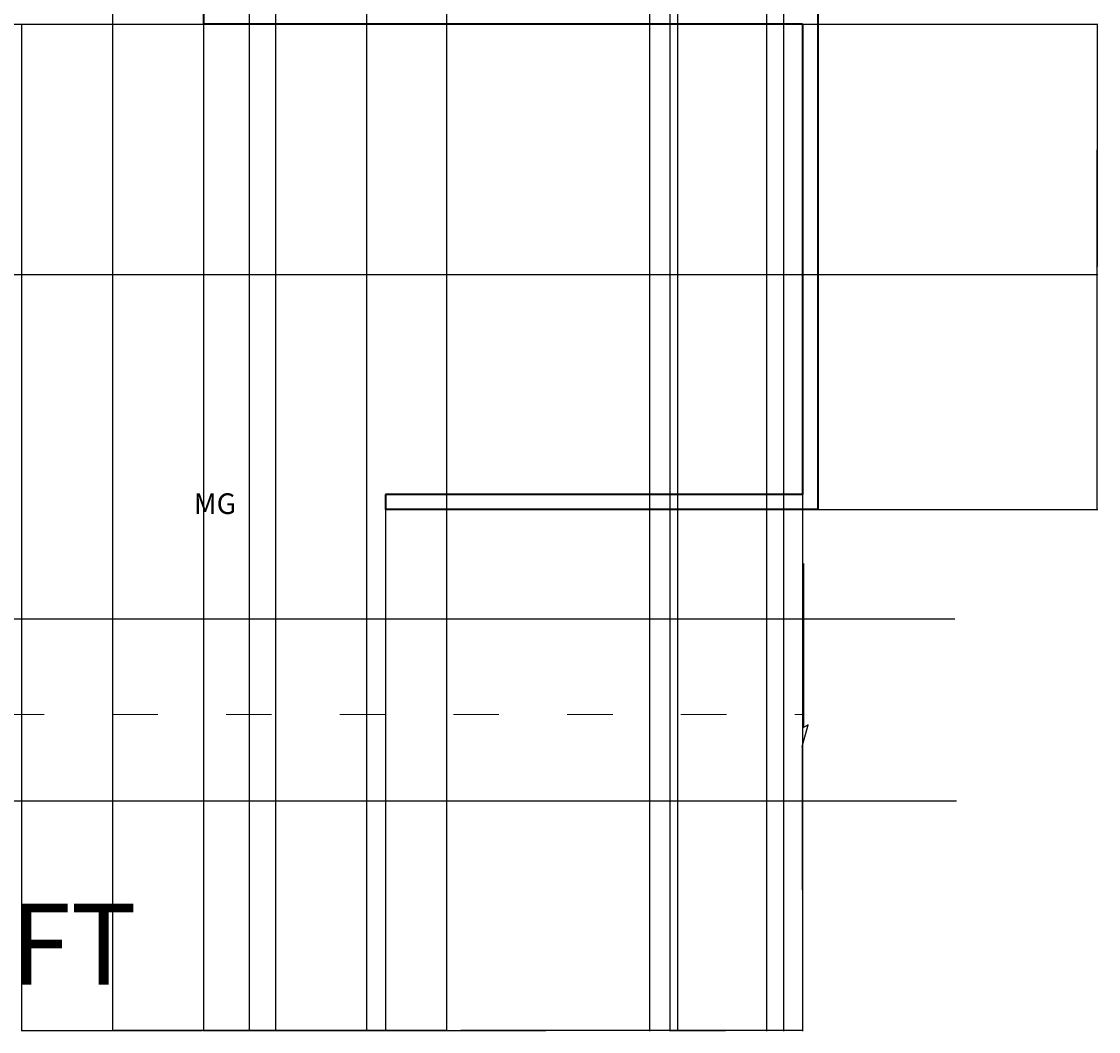
# Model space of a CAD drawing. Units: inches. Extents: x 320 to 1055, y -655 to 96.
# Tile 2 of 4: x 771 to 1055, y -655 to -389. Entities that reach past the tile are written whole.
import ezdxf

# ---------------------------------------------------------------- set-up
doc = ezdxf.new("R2010")
doc.units = ezdxf.units.IN
doc.header["$MEASUREMENT"] = 0
doc.linetypes.add('ACAD_ISO03W100', pattern=[30, 12, -18])
for name, color, linetype, lineweight in [('A-ANNO-DIMS', 2, 'Continuous', 18), ('A-ANNO-IDEN', 1, 'Continuous', 18), ('A-ANNO-TEXT', 8, 'Continuous', 18), ('C-ROAD', 1, 'Continuous', 25), ('C-ROAD-CNTR', 1, 'ACAD_ISO03W100', 18), ('wall', 1, 'Continuous', 35)]:
    doc.layers.add(name, color=color, linetype=linetype, lineweight=lineweight)
doc.styles.get("Standard").update_dxf_attribs({"font": 'arial.ttf'})
doc.dimstyles.get("Standard").update_dxf_attribs({"dimtxt": 0.18, "dimasz": 0.18, "dimexe": 0.18, "dimexo": 0.0625, "dimgap": 0.09, "dimtad": 0, "dimtih": 1, "dimtoh": 1, "dimdec": 1, "dimzin": 0, "dimdsep": 46, "dimlunit": 4, "dimtxsty": 'Standard', "dimcen": 0.09, "dimadec": 0, "dimazin": 0, "dimtfac": 1, "dimtdec": 1, "dimtofl": 0, "dimtmove": 0, "dimatfit": 3, "dimfxl": 1, "dimtolj": 1, "dimtzin": 0, "dimarcsym": 0})

# ---------------------------------------------------------------- blocks, each defined once
blk = doc.blocks.new('*D17')
at = {"layer": 'A-ANNO-DIMS', "color": 0, "lineweight": -2, "transparency": 16777216}
for p, q in [((770.86, -517.8), (770.86, -655.29)), ((866.86, -517.8), (866.86, -655.29)), ((771.04, -655.11), (818.53, -655.11)), ((866.68, -655.11), (819.19, -655.11))]:
    blk.add_line(p, q, dxfattribs=at)
at = {"layer": 'A-ANNO-DIMS', "color": 0, "transparency": 16777216}
for points in [[(771.04, -655.08), (771.04, -655.14), (770.86, -655.11)], [(866.68, -655.08), (866.68, -655.14), (866.86, -655.11)]]:
    blk.add_solid(points, dxfattribs=at)
at = {"layer": 'Defpoints', "color": 0, "transparency": 16777216}
for p in [(770.86, -517.74), (866.86, -517.74), (866.86, -655.11)]:
    blk.add_point(p, dxfattribs=at)
at = {"layer": 'A-ANNO-DIMS', "color": 0, "transparency": 16777216, "insert": (818.86, -655.11), "char_height": 0.18, "attachment_point": 5}
blk.add_mtext('\\A1;8\'-0"', dxfattribs=at)
blk = doc.blocks.new('*D18')
at = {"layer": 'A-ANNO-DIMS', "color": 0, "lineweight": -2, "transparency": 16777216}
for p, q in [((818.86, -389.8), (818.86, -655.29)), ((976.86, -389.8), (976.86, -655.29)), ((819.04, -655.11), (897.47, -655.11)), ((976.68, -655.11), (898.25, -655.11))]:
    blk.add_line(p, q, dxfattribs=at)
at = {"layer": 'A-ANNO-DIMS', "color": 0, "transparency": 16777216}
for points in [[(819.04, -655.08), (819.04, -655.14), (818.86, -655.11)], [(976.68, -655.08), (976.68, -655.14), (976.86, -655.11)]]:
    blk.add_solid(points, dxfattribs=at)
at = {"layer": 'Defpoints', "color": 0, "transparency": 16777216}
for p in [(818.86, -389.74), (976.86, -389.74), (976.86, -655.11)]:
    blk.add_point(p, dxfattribs=at)
at = {"layer": 'A-ANNO-DIMS', "color": 0, "transparency": 16777216, "insert": (897.86, -655.11), "char_height": 0.18, "attachment_point": 5}
blk.add_mtext('\\A1;13\'-2"', dxfattribs=at)
blk = doc.blocks.new('*D19')
at = {"layer": 'A-ANNO-DIMS', "color": 0, "lineweight": -2, "transparency": 16777216}
for p, q in [((976.92, -389.74), (1054.75, -389.74)), ((1054.57, -389.92), (1054.57, -453.55)), ((1054.57, -517.56), (1054.57, -453.92)), ((980.92, -517.74), (1054.75, -517.74))]:
    blk.add_line(p, q, dxfattribs=at)
at = {"layer": 'A-ANNO-DIMS', "color": 0, "transparency": 16777216}
for points in [[(1054.54, -389.92), (1054.6, -389.92), (1054.57, -389.74)], [(1054.54, -517.56), (1054.6, -517.56), (1054.57, -517.74)]]:
    blk.add_solid(points, dxfattribs=at)
at = {"layer": 'Defpoints', "color": 0, "transparency": 16777216}
for p in [(976.86, -389.74), (980.86, -517.74), (1054.57, -517.74)]:
    blk.add_point(p, dxfattribs=at)
at = {"layer": 'A-ANNO-DIMS', "color": 0, "transparency": 16777216, "insert": (1054.57, -453.74), "char_height": 0.18, "attachment_point": 5}
blk.add_mtext('\\A1;10\'-8"', dxfattribs=at)
blk = doc.blocks.new('*D20')
at = {"layer": 'A-ANNO-DIMS', "color": 0, "lineweight": -2, "transparency": 16777216}
for p, q in [((770.86, -389.8), (770.86, -655.29)), ((818.86, -389.8), (818.86, -655.29)), ((771.04, -655.11), (794.53, -655.11)), ((818.68, -655.11), (795.19, -655.11))]:
    blk.add_line(p, q, dxfattribs=at)
at = {"layer": 'A-ANNO-DIMS', "color": 0, "transparency": 16777216}
for points in [[(771.04, -655.08), (771.04, -655.14), (770.86, -655.11)], [(818.68, -655.08), (818.68, -655.14), (818.86, -655.11)]]:
    blk.add_solid(points, dxfattribs=at)
at = {"layer": 'Defpoints', "color": 0, "transparency": 16777216}
for p in [(770.86, -389.74), (818.86, -389.74), (818.86, -655.11)]:
    blk.add_point(p, dxfattribs=at)
at = {"layer": 'A-ANNO-DIMS', "color": 0, "transparency": 16777216, "insert": (794.86, -655.11), "char_height": 0.18, "attachment_point": 5}
blk.add_mtext('\\A1;4\'-0"', dxfattribs=at)
blk = doc.blocks.new('*D23')
at = {"layer": 'A-ANNO-DIMS', "color": 0, "lineweight": -2, "transparency": 16777216}
for p, q in [((794.86, -80.8), (794.86, -655.29)), ((818.86, -80.8), (818.86, -655.29)), ((795.04, -655.11), (806.53, -655.11)), ((818.68, -655.11), (807.19, -655.11))]:
    blk.add_line(p, q, dxfattribs=at)
at = {"layer": 'A-ANNO-DIMS', "color": 0, "transparency": 16777216}
for points in [[(795.04, -655.08), (795.04, -655.14), (794.86, -655.11)], [(818.68, -655.08), (818.68, -655.14), (818.86, -655.11)]]:
    blk.add_solid(points, dxfattribs=at)
at = {"layer": 'Defpoints', "color": 0, "transparency": 16777216}
for p in [(794.86, -80.74), (818.86, -80.74), (818.86, -655.11)]:
    blk.add_point(p, dxfattribs=at)
at = {"layer": 'A-ANNO-DIMS', "color": 0, "transparency": 16777216, "insert": (806.86, -655.11), "char_height": 0.18, "attachment_point": 5}
blk.add_mtext('\\A1;2\'-0"', dxfattribs=at)
blk = doc.blocks.new('*D25')
at = {"layer": 'A-ANNO-DIMS', "color": 0, "lineweight": -2, "transparency": 16777216}
for p, q in [((941.86, -380.8), (941.86, -655.29)), ((971.86, -380.8), (971.86, -655.29)), ((942.04, -655.11), (956.53, -655.11)), ((971.68, -655.11), (957.19, -655.11))]:
    blk.add_line(p, q, dxfattribs=at)
at = {"layer": 'A-ANNO-DIMS', "color": 0, "transparency": 16777216}
for points in [[(942.04, -655.08), (942.04, -655.14), (941.86, -655.11)], [(971.68, -655.08), (971.68, -655.14), (971.86, -655.11)]]:
    blk.add_solid(points, dxfattribs=at)
at = {"layer": 'Defpoints', "color": 0, "transparency": 16777216}
for p in [(941.86, -380.74), (971.86, -380.74), (941.86, -655.11)]:
    blk.add_point(p, dxfattribs=at)
at = {"layer": 'A-ANNO-DIMS', "color": 0, "transparency": 16777216, "insert": (956.86, -655.11), "char_height": 0.18, "attachment_point": 5}
blk.add_mtext('\\A1;2\'-6"', dxfattribs=at)
blk = doc.blocks.new('*D28')
at = {"layer": 'A-ANNO-DIMS', "color": 0, "lineweight": -2, "transparency": 16777216}
for p, q in [((943.86, -363.86), (943.86, -655.29)), ((967.33, -363.86), (967.33, -655.29)), ((944.04, -655.11), (955, -655.11)), ((967.15, -655.11), (956.2, -655.11))]:
    blk.add_line(p, q, dxfattribs=at)
at = {"layer": 'A-ANNO-DIMS', "color": 0, "transparency": 16777216}
for points in [[(944.04, -655.08), (944.04, -655.14), (943.86, -655.11)], [(967.15, -655.08), (967.15, -655.14), (967.33, -655.11)]]:
    blk.add_solid(points, dxfattribs=at)
at = {"layer": 'Defpoints', "color": 0, "transparency": 16777216}
for p in [(943.86, -363.79), (967.33, -363.79), (967.33, -655.11)]:
    blk.add_point(p, dxfattribs=at)
at = {"layer": 'A-ANNO-DIMS', "color": 0, "transparency": 16777216, "insert": (955.6, -655.11), "char_height": 0.18, "attachment_point": 5}
blk.add_mtext('\\A1;1\'-11 1/2"', dxfattribs=at)
blk = doc.blocks.new('*D30')
at = {"layer": 'A-ANNO-DIMS', "color": 0, "lineweight": -2, "transparency": 16777216}
for p, q in [((837.86, -248.8), (837.86, -655.29)), ((861.86, -248.8), (861.86, -655.29)), ((838.04, -655.11), (849.53, -655.11)), ((861.68, -655.11), (850.19, -655.11))]:
    blk.add_line(p, q, dxfattribs=at)
at = {"layer": 'A-ANNO-DIMS', "color": 0, "transparency": 16777216}
for points in [[(838.04, -655.08), (838.04, -655.14), (837.86, -655.11)], [(861.68, -655.08), (861.68, -655.14), (861.86, -655.11)]]:
    blk.add_solid(points, dxfattribs=at)
at = {"layer": 'Defpoints', "color": 0, "transparency": 16777216}
for p in [(837.86, -248.74), (861.86, -248.74), (861.86, -655.11)]:
    blk.add_point(p, dxfattribs=at)
at = {"layer": 'A-ANNO-DIMS', "color": 0, "transparency": 16777216, "insert": (849.86, -655.11), "char_height": 0.18, "attachment_point": 5}
blk.add_mtext('\\A1;2\'-0"', dxfattribs=at)
blk = doc.blocks.new('*D31')
at = {"layer": 'A-ANNO-DIMS', "color": 0, "lineweight": -2, "transparency": 16777216}
for p, q in [((882.91, -200.15), (882.91, -655.29)), ((936.46, -200.15), (936.46, -655.29)), ((883.09, -655.11), (909.14, -655.11)), ((936.28, -655.11), (910.23, -655.11))]:
    blk.add_line(p, q, dxfattribs=at)
at = {"layer": 'A-ANNO-DIMS', "color": 0, "transparency": 16777216}
for points in [[(883.09, -655.08), (883.09, -655.14), (882.91, -655.11)], [(936.28, -655.08), (936.28, -655.14), (936.46, -655.11)]]:
    blk.add_solid(points, dxfattribs=at)
at = {"layer": 'Defpoints', "color": 0, "transparency": 16777216}
for p in [(882.91, -200.08), (936.46, -200.08), (936.46, -655.11)]:
    blk.add_point(p, dxfattribs=at)
at = {"layer": 'A-ANNO-DIMS', "color": 0, "transparency": 16777216, "insert": (909.68, -655.11), "char_height": 0.18, "attachment_point": 5}
blk.add_mtext('\\A1;4\'-5 1/2"', dxfattribs=at)
blk = doc.blocks.new('*D34')
at = {"layer": 'A-ANNO-DIMS', "color": 0, "lineweight": -2, "transparency": 16777216}
for p, q in [((556.92, -389.74), (1054.75, -389.74)), ((1054.57, -389.92), (1054.57, -422.55)), ((1054.57, -455.56), (1054.57, -422.92)), ((556.92, -455.74), (1054.75, -455.74))]:
    blk.add_line(p, q, dxfattribs=at)
at = {"layer": 'A-ANNO-DIMS', "color": 0, "transparency": 16777216}
for points in [[(1054.54, -389.92), (1054.6, -389.92), (1054.57, -389.74)], [(1054.54, -455.56), (1054.6, -455.56), (1054.57, -455.74)]]:
    blk.add_solid(points, dxfattribs=at)
at = {"layer": 'Defpoints', "color": 0, "transparency": 16777216}
for p in [(556.86, -389.74), (556.86, -455.74), (1054.57, -455.74)]:
    blk.add_point(p, dxfattribs=at)
at = {"layer": 'A-ANNO-DIMS', "color": 0, "transparency": 16777216, "insert": (1054.57, -422.74), "char_height": 0.18, "attachment_point": 5}
blk.add_mtext('\\A1;5\'-6"', dxfattribs=at)
blk = doc.blocks.new('*D54')
at = {"layer": 'A-ANNO-DIMS', "color": 0, "lineweight": -2, "transparency": 16777216}
for p, q in [((882.91, -200.15), (882.91, -655.29)), ((830.86, -231.8), (830.86, -655.29)), ((831.04, -655.11), (856.55, -655.11)), ((882.73, -655.11), (857.22, -655.11))]:
    blk.add_line(p, q, dxfattribs=at)
at = {"layer": 'A-ANNO-DIMS', "color": 0, "transparency": 16777216}
for points in [[(831.04, -655.08), (831.04, -655.14), (830.86, -655.11)], [(882.73, -655.08), (882.73, -655.14), (882.91, -655.11)]]:
    blk.add_solid(points, dxfattribs=at)
at = {"layer": 'Defpoints', "color": 0, "transparency": 16777216}
for p in [(882.91, -200.08), (830.86, -231.74), (882.91, -655.11)]:
    blk.add_point(p, dxfattribs=at)
at = {"layer": 'A-ANNO-DIMS', "color": 0, "transparency": 16777216, "insert": (856.89, -655.11), "char_height": 0.18, "attachment_point": 5}
blk.add_mtext('\\A1;4\'-4"', dxfattribs=at)
blk = doc.blocks.new('*D56')
at = {"layer": 'A-ANNO-DIMS', "color": 0, "lineweight": -2, "transparency": 16777216}
for p, q in [((830.86, -380.8), (830.86, -655.29)), ((941.86, -380.8), (941.86, -655.29)), ((831.04, -655.11), (886.03, -655.11)), ((941.68, -655.11), (886.69, -655.11))]:
    blk.add_line(p, q, dxfattribs=at)
at = {"layer": 'A-ANNO-DIMS', "color": 0, "transparency": 16777216}
for points in [[(831.04, -655.08), (831.04, -655.14), (830.86, -655.11)], [(941.68, -655.08), (941.68, -655.14), (941.86, -655.11)]]:
    blk.add_solid(points, dxfattribs=at)
at = {"layer": 'Defpoints', "color": 0, "transparency": 16777216}
for p in [(830.86, -380.74), (941.86, -380.74), (941.86, -655.11)]:
    blk.add_point(p, dxfattribs=at)
at = {"layer": 'A-ANNO-DIMS', "color": 0, "transparency": 16777216, "insert": (886.36, -655.11), "char_height": 0.18, "attachment_point": 5}
blk.add_mtext('\\A1;9\'-3"', dxfattribs=at)

msp = doc.modelspace()

# ---------------------------------------------------------------- linework, layer by layer
at = {"layer": 'C-ROAD'}
for p, q in [((977.07, -531.93), (977.07, -575.22)), ((357.35, -546.58), (1017.02, -546.58)), ((976.72, -580.26), (978.38, -574.53)), ((978.38, -574.53), (977.07, -575.22)), ((976.72, -579.95), (976.72, -617.98)), ((357.35, -594.58), (1017.44, -594.58))]:
    msp.add_line(p, q, dxfattribs=at)
at = {"layer": 'C-ROAD-CNTR'}
msp.add_line((674.79, -571.77), (976.72, -571.77), dxfattribs=at)
at = {"layer": 'wall'}
for p, q in [((980.86, 10.26), (980.86, -517.74)), ((818.86, -380.74), (818.86, -389.74)), ((976.86, -389.74), (818.86, -389.74)), ((976.86, -389.74), (976.86, -513.74)), ((872.86, -513.74), (866.86, -513.74)), ((866.86, -513.74), (866.86, -517.74)), ((976.86, -513.74), (872.86, -513.74)), ((872.86, -517.74), (866.86, -517.74)), ((872.86, -517.74), (866.86, -517.74)), ((980.86, -517.74), (872.86, -517.74)), ((980.86, -517.74), (944.86, -517.74))]:
    msp.add_line(p, q, dxfattribs=at)

# ---------------------------------------------------------------- texts
at = {"layer": 'A-ANNO-IDEN'}
msp.add_text('MG', height=5.444, dxfattribs=at).set_placement((816.29, -518.89))
at = {"layer": 'A-ANNO-TEXT', "insert": (571.05, -621.71), "char_height": 21.2807, "attachment_point": 1}
msp.add_mtext_dynamic_manual_height_columns('AREA=1936 SQFT', width=263.9184, gutter_width=3.55, heights=[0], dxfattribs=at)

# ---------------------------------------------------------------- dimensions: what is measured, and where the dimension line sits
at = {"layer": 'A-ANNO-DIMS'}
for base, p1, p2, picture, middle in [((818.86, -655.11), (794.86, -80.74), (818.86, -80.74), '*D23', (806.86, -655.11)), ((882.9112, -655.1081), (830.8589, -231.7361), (882.9112, -200.0844), '*D54', (856.885, -655.1081)), ((936.4561, -655.1081), (882.9112, -200.0844), (936.4561, -200.0844), '*D31', (909.6836, -655.1081)), ((861.86, -655.11), (837.86, -248.74), (861.86, -248.74), '*D30', (849.86, -655.11)), ((967.33, -655.11), (943.86, -363.79), (967.33, -363.79), '*D28', (955.6, -655.11)), ((941.86, -655.11), (830.86, -380.74), (941.86, -380.74), '*D56', (886.36, -655.11)), ((941.86, -655.11), (971.86, -380.74), (941.86, -380.74), '*D25', (956.86, -655.11)), ((818.86, -655.11), (770.86, -389.74), (818.86, -389.74), '*D20', (794.86, -655.11)), ((976.86, -655.11), (818.86, -389.74), (976.86, -389.74), '*D18', (897.86, -655.11)), ((866.86, -655.11), (770.86, -517.74), (866.86, -517.74), '*D17', (818.86, -655.11))]:
    dim = msp.add_linear_dim(base=base, p1=p1, p2=p2, dimstyle='Standard', override={"dimdec": 1, "dimlfac": 1, "dimrnd": 0, "dimzin": 1, "dimdsep": 46, "dimlunit": 4, "dimfrac": 2}, dxfattribs=at)
    dim.commit()
    dim.dimension.update_dxf_attribs({"geometry": picture, "text_midpoint": middle})
for base, p1, p2, picture, middle in [((1054.57, -455.74), (556.86, -389.74), (556.86, -455.74), '*D34', (1054.57, -422.74)), ((1054.57, -517.74), (976.86, -389.74), (980.86, -517.74), '*D19', (1054.57, -453.74))]:
    dim = msp.add_linear_dim(base=base, p1=p1, p2=p2, angle=90, dimstyle='Standard', override={"dimdec": 1, "dimlfac": 1, "dimrnd": 0, "dimzin": 1, "dimdsep": 46, "dimlunit": 4, "dimfrac": 2}, dxfattribs=at)
    dim.commit()
    dim.dimension.update_dxf_attribs({"geometry": picture, "text_midpoint": middle})

doc.saveas('drawing.dxf')
